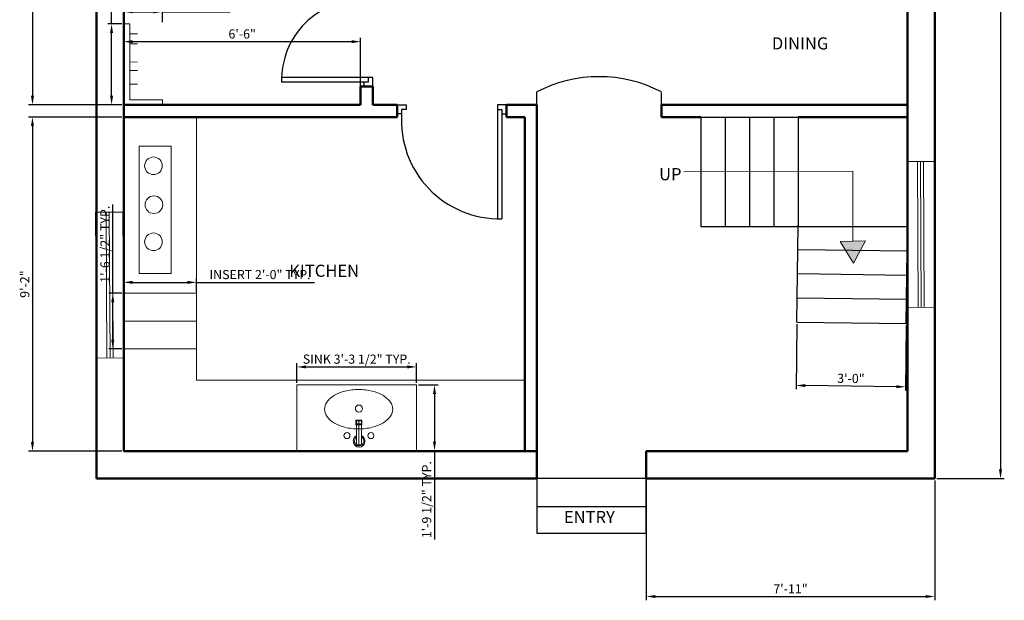
# Model space of a CAD drawing. Units: inches. Extents: x 108 to 1546, y -229 to 513.
# Tile 1 of 11: x 108 to 432, y -44 to 147. Entities that reach past the tile are written whole.
import ezdxf

# ---------------------------------------------------------------- set-up
doc = ezdxf.new("R2010")
doc.units = ezdxf.units.IN
for name, color, linetype, lineweight in [('A-ANNO-DIMS', 2, 'Continuous', 18), ('A-ANNO-SYMB', 4, 'Continuous', 18), ('A-AREA-IDEN', 4, 'Continuous', 18), ('A-EQPM', 8, 'Continuous', 18), ('A-FLOR-CBNT', 8, 'Continuous', 18), ('A-FLOR-FIXT', 9, 'Continuous', 18), ('A-FLOR-STRS', 7, 'Continuous', 25), ('door', 1, 'Continuous', 25), ('wall', 7, 'Continuous', 50), ('WINDOW', 212, 'Continuous', 18)]:
    doc.layers.add(name, color=color, linetype=linetype, lineweight=lineweight)
doc.styles.get("Standard").update_dxf_attribs({"font": 'arial.ttf'})
doc.dimstyles.new('ISO-25', dxfattribs={"dimtxt": 3, "dimasz": 3, "dimexe": 1.25, "dimexo": 0.625, "dimtad": 1, "dimdec": 1, "dimlunit": 3, "dimtxsty": 'Standard', "dimcen": 2.5, "dimadec": 0, "dimazin": 0, "dimtfac": 1, "dimtdec": 1, "dimtmove": 0, "dimatfit": 3, "dimfxl": 1, "dimarcsym": 0})

# ---------------------------------------------------------------- blocks, each defined once
blk = doc.blocks.new('A$C50A015BB')
for p, q in [((0, 0.55), (1, 0.55)), ((0, 0.55), (0, 0)), ((0.4985, 0.5), (0.5385, 0.5)), ((0.4985, 0.5), (0.4985, 0.3)), ((0.5185, 0.5), (0.5185, 0.3)), ((0.5385, 0.5), (0.5385, 0.3)), ((1, 0.55), (1, 0)), ((0.4935, 0.335), (0.4935, 0.295)), ((0.4935, 0.335), (0.5435, 0.335)), ((0.5435, 0.335), (0.5435, 0.295)), ((0.4935, 0.295), (0.5435, 0.295)), ((0.4985, 0.325), (0.5385, 0.325)), ((0.4985, 0.3), (0.5385, 0.3)), ((0, 0), (1, 0)), ((0, 0), (1, 0))]:
    blk.add_line(p, q)
for centre, radius in [((0.4185, 0.424), 0.025), ((0.6185, 0.424), 0.025), ((0.5185, 0.1981), 0.0298)]:
    blk.add_circle(centre, radius)
for centre, radius, start, end in [((0.5201, 0.4703), 0.0497, 291.74253, 244.23308), ((0.5201, 0.4703), 0.0397, 297.63203, 237.02558), ((0.4772, 0.0383), 0.3252, 103.48533, 120.06859), ((0.5157, -0.1225), 0.4906, 90, 103.48533), ((0.5157, -0.1225), 0.4906, 76.51467, 90), ((0.5543, 0.0383), 0.3252, 59.93141, 76.51467), ((0.3299, 0.2031), 0.0991, 144.41781, 180), ((0.4185, 0.1397), 0.2081, 120.06859, 144.41781), ((0.613, 0.1397), 0.2081, 35.58219, 59.93141), ((0.7016, 0.2031), 0.0991, 0, 35.58219), ((0.3299, 0.2031), 0.0991, 180, 215.58219), ((0.7016, 0.2031), 0.0991, 324.41781, 0), ((0.4185, 0.2665), 0.2081, 215.58219, 239.93141), ((0.4772, 0.3679), 0.3252, 239.93141, 256.51467), ((0.5543, 0.3679), 0.3252, 283.48533, 300.06859), ((0.613, 0.2665), 0.2081, 300.06859, 324.41781), ((0.5157, 0.5288), 0.4906, 256.51467, 270), ((0.5157, 0.5288), 0.4906, 270, 283.48533)]:
    blk.add_arc(centre, radius, start, end)
blk = doc.blocks.new('*D22')
at = {"layer": 'A-ANNO-DIMS', "color": 0, "lineweight": -2, "transparency": 16777216}
for p, q in [((409.55, 356.47), (431.8, 356.47)), ((430.55, 353.47), (430.55, -0.53)), ((409.55, -3.53), (431.8, -3.53))]:
    blk.add_line(p, q, dxfattribs=at)
at = {"layer": 'A-ANNO-DIMS', "color": 0, "transparency": 16777216}
for points in [[(430.05, 353.47), (431.05, 353.47), (430.55, 356.47)], [(430.05, -0.53), (431.05, -0.53), (430.55, -3.53)]]:
    blk.add_solid(points, dxfattribs=at)
at = {"layer": 'Defpoints', "color": 0, "transparency": 16777216}
for p in [(408.92, 356.47), (408.92, -3.53), (430.55, -3.53)]:
    blk.add_point(p, dxfattribs=at)
at = {"layer": 'A-ANNO-DIMS', "color": 0, "transparency": 16777216, "insert": (428.39, 176.47), "char_height": 3, "attachment_point": 5, "rotation": 90}
blk.add_mtext("30'", dxfattribs=at)
blk = doc.blocks.new('WINDOW-48X9')
for p, q in [((0, 9), (0, 0)), ((0, 9), (48, 9)), ((48, 9), (48, 0)), ((0, 5.5), (48, 5.5)), ((0, 4.5), (48, 4.5)), ((0, 3.5), (48, 3.5)), ((0, 0), (48, 0))]:
    blk.add_line(p, q)
blk = doc.blocks.new('DOOR-SWING-36')
for p, q in [((1.5, 1.5), (1.5, 37.5)), ((3, 1.5), (3, 37.5)), ((0, 3), (0, 0)), ((1.5, 3), (0, 3)), ((1.5, 1.5), (1.5, 3)), ((3, 1.5), (1.5, 1.5)), ((3, 0), (3, 1.5)), ((33, 0), (33, 1.5)), ((33, 1.5), (34.5, 1.5)), ((34.5, 1.5), (34.5, 3)), ((34.5, 3), (36, 3)), ((36, 3), (36, 0)), ((0, 0), (3, 0)), ((36, 0), (33, 0))]:
    blk.add_line(p, q)
blk.add_arc((2.25, 5.18), 32.32, 356.1244, 91.3295)
blk = doc.blocks.new('DOOR-SWING-30')
for p, q in [((27, 30), (30, 30)), ((27, 28.5), (27, 30)), ((30, 30), (30, 27)), ((28.5, 28.5), (27, 28.5)), ((28.5, 27), (28.5, 28.5)), ((30, 27), (28.5, 27)), ((30, 3), (0, 3)), ((28.5, 1.5), (0, 1.5)), ((28.5, 1.5), (27, 1.5)), ((27, 1.5), (27, 0)), ((30, 3), (28.5, 3)), ((28.5, 3), (28.5, 1.5)), ((30, 0), (30, 3)), ((27, 0), (30, 0))]:
    blk.add_line(p, q)
blk.add_arc((26.25, 2.25), 26.26, 88.3634, 181.6366)
blk = doc.blocks.new('COOKTOP-3-BURNER')
blk.add_lwpolyline([(0, 41.89), (10.48, 41.89), (10.48, 0), (0, 0)], close=True)
for centre in [(4.66, 35.46), (4.81, 22.66), (4.66, 10.45)]:
    blk.add_circle(centre, 2.9)
blk = doc.blocks.new('COUNTER-INSERT-DIVIDED')
blk.add_line((0, 9.14), (23.96, 9.14))
blk.add_lwpolyline([(0, 18.28), (23.96, 18.28), (23.96, 0), (0, 0)], close=True)
blk = doc.blocks.new('ENTRY-STEPS-36')
for p, q in [((0, 8.79), (36, 8.79)), ((0, 0), (36, 0))]:
    blk.add_line(p, q)
blk.add_lwpolyline([(36, 0), (36, 18), (0, 18), (0, 0)])
blk = doc.blocks.new('BATH-CORNER-RACK')
for p, q in [((2.03, 23.32), (4.51, 23.38)), ((2.03, 20.06), (4.51, 20.12)), ((2.03, 14.08), (4.51, 14.14)), ((2.03, 11.27), (4.51, 11.33)), ((2.03, 6.76), (4.51, 6.83))]:
    blk.add_line(p, q)
for points in [[(2.03, 1.66), (2.03, 26.63), (0, 26.63), (0, 0), (2.03, 0)], [(0, 1.66), (0, 1.66), (0, 0), (12.78, 0), (12.78, 1.66), (2.03, 1.66)]]:
    blk.add_lwpolyline(points)
blk = doc.blocks.new('*D56')
at = {"layer": 'A-ANNO-DIMS', "color": 0, "lineweight": -2, "transparency": 16777216}
for p, q in [((198.95, 27.94), (198.95, 34.47)), ((201.95, 33.22), (235.32, 33.22)), ((238.32, 27.94), (238.32, 34.47))]:
    blk.add_line(p, q, dxfattribs=at)
at = {"layer": 'A-ANNO-DIMS', "color": 0, "transparency": 16777216}
for points in [[(201.95, 33.72), (201.95, 32.72), (198.95, 33.22)], [(235.32, 33.72), (235.32, 32.72), (238.32, 33.22)]]:
    blk.add_solid(points, dxfattribs=at)
at = {"layer": 'Defpoints', "color": 0, "transparency": 16777216}
for p in [(238.32, 33.22), (198.95, 27.31), (238.32, 27.31)]:
    blk.add_point(p, dxfattribs=at)
at = {"layer": 'A-ANNO-DIMS', "color": 0, "transparency": 16777216, "insert": (218.64, 35.39), "char_height": 3, "attachment_point": 5}
blk.add_mtext('SINK 3\'-3 1/2" TYP.', dxfattribs=at)
blk = doc.blocks.new('*D57')
at = {"layer": 'A-ANNO-DIMS', "color": 0, "lineweight": -2, "transparency": 16777216}
for p, q in [((238.95, 27.31), (245.48, 27.31)), ((244.23, 24.31), (244.23, 8.66)), ((238.95, 5.66), (245.48, 5.66)), ((244.23, 5.66), (244.23, -23.59))]:
    blk.add_line(p, q, dxfattribs=at)
at = {"layer": 'A-ANNO-DIMS', "color": 0, "transparency": 16777216}
for points in [[(243.73, 24.31), (244.73, 24.31), (244.23, 27.31)], [(243.73, 8.66), (244.73, 8.66), (244.23, 5.66)]]:
    blk.add_solid(points, dxfattribs=at)
at = {"layer": 'Defpoints', "color": 0, "transparency": 16777216}
for p in [(238.32, 27.31), (238.32, 5.66), (244.23, 5.66)]:
    blk.add_point(p, dxfattribs=at)
at = {"layer": 'A-ANNO-DIMS', "color": 0, "transparency": 16777216, "insert": (242.05, -10.47), "char_height": 3, "attachment_point": 5, "rotation": 90}
blk.add_mtext('1\'-9 1/2" TYP.', dxfattribs=at)
blk = doc.blocks.new('*D64')
at = {"layer": 'A-ANNO-DIMS', "color": 0, "lineweight": -2, "transparency": 16777216}
for p, q in [((141.92, 58.09), (141.92, 62.31)), ((165.89, 58.09), (165.89, 62.31)), ((144.92, 61.06), (162.89, 61.06)), ((165.89, 61.06), (204.74, 61.06))]:
    blk.add_line(p, q, dxfattribs=at)
at = {"layer": 'A-ANNO-DIMS', "color": 0, "transparency": 16777216}
for points in [[(144.92, 61.56), (144.92, 60.56), (141.92, 61.06)], [(162.89, 61.56), (162.89, 60.56), (165.89, 61.06)]]:
    blk.add_solid(points, dxfattribs=at)
at = {"layer": 'Defpoints', "color": 0, "transparency": 16777216}
for p in [(165.89, 61.06), (141.92, 57.46), (165.89, 57.46)]:
    blk.add_point(p, dxfattribs=at)
at = {"layer": 'A-ANNO-DIMS', "color": 0, "transparency": 16777216, "insert": (186.81, 63.23), "char_height": 3, "attachment_point": 5}
blk.add_mtext('INSERT 2\'-0" TYP.', dxfattribs=at)
blk = doc.blocks.new('*D65')
at = {"layer": 'A-ANNO-DIMS', "color": 0, "lineweight": -2, "transparency": 16777216}
for p, q in [((138.33, 57.46), (138.33, 86.71)), ((141.3, 57.46), (137.08, 57.46)), ((138.33, 42.18), (138.33, 54.46)), ((141.3, 39.18), (137.08, 39.18))]:
    blk.add_line(p, q, dxfattribs=at)
at = {"layer": 'A-ANNO-DIMS', "color": 0, "transparency": 16777216}
for points in [[(137.83, 54.46), (138.83, 54.46), (138.33, 57.46)], [(137.83, 42.18), (138.83, 42.18), (138.33, 39.18)]]:
    blk.add_solid(points, dxfattribs=at)
at = {"layer": 'Defpoints', "color": 0, "transparency": 16777216}
for p in [(138.33, 57.46), (141.92, 57.46), (141.92, 39.18)]:
    blk.add_point(p, dxfattribs=at)
at = {"layer": 'A-ANNO-DIMS', "color": 0, "transparency": 16777216, "insert": (136.15, 73.59), "char_height": 3, "attachment_point": 5, "rotation": 90}
blk.add_mtext('1\'-6 1/2" TYP.', dxfattribs=at)
blk = doc.blocks.new('*D68')
at = {"layer": 'A-ANNO-DIMS', "color": 0, "lineweight": -2, "transparency": 16777216}
for p, q in [((137.93, 146.1), (137.93, 188.28)), ((141.3, 146.1), (136.68, 146.1)), ((137.93, 122.47), (137.93, 143.1)), ((141.3, 119.47), (136.68, 119.47))]:
    blk.add_line(p, q, dxfattribs=at)
at = {"layer": 'A-ANNO-DIMS', "color": 0, "transparency": 16777216}
for points in [[(137.43, 143.1), (138.43, 143.1), (137.93, 146.1)], [(137.43, 122.47), (138.43, 122.47), (137.93, 119.47)]]:
    blk.add_solid(points, dxfattribs=at)
at = {"layer": 'Defpoints', "color": 0, "transparency": 16777216}
for p in [(137.93, 146.1), (141.92, 146.1), (141.92, 119.47)]:
    blk.add_point(p, dxfattribs=at)
at = {"layer": 'A-ANNO-DIMS', "color": 0, "transparency": 16777216, "insert": (135.75, 168.69), "char_height": 3, "attachment_point": 5, "rotation": 90}
blk.add_mtext('RACK 2\'-2 1/2" TYP.', dxfattribs=at)
blk = doc.blocks.new('*D69')
at = {"layer": 'A-ANNO-DIMS', "color": 0, "lineweight": -2, "transparency": 16777216}
for p, q in [((141.92, 146.72), (141.92, 151.34)), ((144.92, 150.09), (151.7, 150.09)), ((154.7, 146.72), (154.7, 151.34)), ((154.7, 150.09), (176.96, 150.09))]:
    blk.add_line(p, q, dxfattribs=at)
at = {"layer": 'A-ANNO-DIMS', "color": 0, "transparency": 16777216}
for points in [[(144.92, 150.59), (144.92, 149.59), (141.92, 150.09)], [(151.7, 150.59), (151.7, 149.59), (154.7, 150.09)]]:
    blk.add_solid(points, dxfattribs=at)
at = {"layer": 'Defpoints', "color": 0, "transparency": 16777216}
for p in [(154.7, 150.09), (141.92, 146.1), (154.7, 146.1)]:
    blk.add_point(p, dxfattribs=at)
at = {"layer": 'A-ANNO-DIMS', "color": 0, "transparency": 16777216, "insert": (167.33, 152.22), "char_height": 3, "attachment_point": 5}
blk.add_mtext('1\'-1" TYP.', dxfattribs=at)
blk = doc.blocks.new('*D74')
at = {"layer": 'A-ANNO-DIMS', "color": 0, "lineweight": -2, "transparency": 16777216}
for p, q in [((141.92, 120.09), (141.92, 141.52)), ((144.92, 140.27), (216.92, 140.27)), ((219.92, 120.09), (219.92, 141.52))]:
    blk.add_line(p, q, dxfattribs=at)
at = {"layer": 'A-ANNO-DIMS', "color": 0, "transparency": 16777216}
for points in [[(144.92, 140.77), (144.92, 139.77), (141.92, 140.27)], [(216.92, 140.77), (216.92, 139.77), (219.92, 140.27)]]:
    blk.add_solid(points, dxfattribs=at)
at = {"layer": 'Defpoints', "color": 0, "transparency": 16777216}
for p in [(219.92, 140.27), (141.92, 119.47), (219.92, 119.47)]:
    blk.add_point(p, dxfattribs=at)
at = {"layer": 'A-ANNO-DIMS', "color": 0, "transparency": 16777216, "insert": (180.92, 142.43), "char_height": 3, "attachment_point": 5}
blk.add_mtext('6\'-6"', dxfattribs=at)
blk = doc.blocks.new('*D75')
at = {"layer": 'A-ANNO-DIMS', "color": 0, "lineweight": -2, "transparency": 16777216}
for p, q in [((313.92, -4.16), (313.92, -43.58)), ((408.92, -4.16), (408.92, -43.58)), ((316.92, -42.33), (405.92, -42.33))]:
    blk.add_line(p, q, dxfattribs=at)
at = {"layer": 'A-ANNO-DIMS', "color": 0, "transparency": 16777216}
for points in [[(316.92, -41.83), (316.92, -42.83), (313.92, -42.33)], [(405.92, -41.83), (405.92, -42.83), (408.92, -42.33)]]:
    blk.add_solid(points, dxfattribs=at)
at = {"layer": 'Defpoints', "color": 0, "transparency": 16777216}
for p in [(313.92, -3.53), (408.92, -3.53), (408.92, -42.33)]:
    blk.add_point(p, dxfattribs=at)
at = {"layer": 'A-ANNO-DIMS', "color": 0, "transparency": 16777216, "insert": (361.42, -40.2), "char_height": 3, "attachment_point": 5}
blk.add_mtext('7\'-11"', dxfattribs=at)
blk = doc.blocks.new('*D77')
at = {"layer": 'A-ANNO-DIMS', "color": 0, "lineweight": -2, "transparency": 16777216}
for p, q in [((141.3, 211.47), (110.64, 211.47)), ((111.89, 208.47), (111.89, 122.47)), ((141.3, 119.47), (110.64, 119.47))]:
    blk.add_line(p, q, dxfattribs=at)
at = {"layer": 'A-ANNO-DIMS', "color": 0, "transparency": 16777216}
for points in [[(111.39, 208.47), (112.39, 208.47), (111.89, 211.47)], [(111.39, 122.47), (112.39, 122.47), (111.89, 119.47)]]:
    blk.add_solid(points, dxfattribs=at)
at = {"layer": 'Defpoints', "color": 0, "transparency": 16777216}
for p in [(141.92, 211.47), (111.89, 119.47), (141.92, 119.47)]:
    blk.add_point(p, dxfattribs=at)
at = {"layer": 'A-ANNO-DIMS', "color": 0, "transparency": 16777216, "insert": (109.73, 165.47), "char_height": 3, "attachment_point": 5, "rotation": 90}
blk.add_mtext('7\'-8"', dxfattribs=at)
blk = doc.blocks.new('*D78')
at = {"layer": 'A-ANNO-DIMS', "color": 0, "lineweight": -2, "transparency": 16777216}
for p, q in [((141.3, 115.47), (110.64, 115.47)), ((111.89, 112.47), (111.89, 8.47)), ((141.3, 5.47), (110.64, 5.47))]:
    blk.add_line(p, q, dxfattribs=at)
at = {"layer": 'A-ANNO-DIMS', "color": 0, "transparency": 16777216}
for points in [[(111.39, 112.47), (112.39, 112.47), (111.89, 115.47)], [(111.39, 8.47), (112.39, 8.47), (111.89, 5.47)]]:
    blk.add_solid(points, dxfattribs=at)
at = {"layer": 'Defpoints', "color": 0, "transparency": 16777216}
for p in [(141.92, 115.47), (111.89, 5.47), (141.92, 5.47)]:
    blk.add_point(p, dxfattribs=at)
at = {"layer": 'A-ANNO-DIMS', "color": 0, "transparency": 16777216, "insert": (109.73, 60.47), "char_height": 3, "attachment_point": 5, "rotation": 90}
blk.add_mtext('9\'-2"', dxfattribs=at)
blk = doc.blocks.new('*D79')
at = {"layer": 'A-ANNO-DIMS', "color": 0, "lineweight": -2, "transparency": 16777216}
for p, q in [((363.52, 47.29), (363.26, 25.87)), ((399.52, 46.85), (399.25, 25.42)), ((396.27, 26.71), (366.27, 27.08))]:
    blk.add_line(p, q, dxfattribs=at)
at = {"layer": 'A-ANNO-DIMS', "color": 0, "transparency": 16777216}
for points in [[(366.28, 27.58), (366.27, 26.58), (363.27, 27.12)], [(396.28, 27.21), (396.26, 26.21), (399.27, 26.67)]]:
    blk.add_solid(points, dxfattribs=at)
at = {"layer": 'Defpoints', "color": 0, "transparency": 16777216}
for p in [(363.53, 47.92), (399.53, 47.47), (363.27, 27.12)]:
    blk.add_point(p, dxfattribs=at)
at = {"layer": 'A-ANNO-DIMS', "color": 0, "transparency": 16777216, "insert": (381.3, 29.05), "char_height": 3, "attachment_point": 5, "rotation": 359.2923}
blk.add_mtext('3\'-0"', dxfattribs=at)

msp = doc.modelspace()

# ---------------------------------------------------------------- hatches: boundary and pattern name
at = {"layer": 'A-ANNO-SYMB'}
h = msp.add_hatch(color=256, dxfattribs=at)
h.dxf.hatch_style = 1
h.paths.add_polyline_path([(386.1, 74.76), (377.74, 74.46), (379.46, 71.72), (384.46, 71.66)])
h.paths.add_polyline_path([(384.46, 71.66), (379.46, 71.72), (382.19, 67.37)])

# ---------------------------------------------------------------- linework, layer by layer
for p, q in [((326.29, 97.47), (381.92, 97.65)), ((381.92, 97.65), (381.92, 74.61))]:
    msp.add_line(p, q, dxfattribs=at)
msp.add_lwpolyline([(382.19, 67.37), (386.1, 74.76), (377.74, 74.46)], close=True, dxfattribs=at)
at = {"layer": 'A-FLOR-CBNT'}
for p, q in [((141.92, 115.47), (165.89, 115.47)), ((141.92, 5.47), (141.92, 115.47)), ((165.89, 115.47), (165.89, 28.9)), ((141.92, 28.9), (141.92, 5.47)), ((273.92, 28.9), (165.89, 28.9)), ((273.92, 5.47), (273.92, 28.9)), ((165.89, 5.47), (141.92, 5.47)), ((141.92, 5.47), (273.92, 5.47))]:
    msp.add_line(p, q, dxfattribs=at)
at = {"layer": 'A-FLOR-FIXT'}
msp.add_line((143.95, 142.79), (143.95, 142.79), dxfattribs=at)
at = {"layer": 'A-FLOR-STRS'}
for p, q in [((331.92, 115.47), (331.92, 79.47)), ((331.92, 115.47), (363.92, 115.47)), ((339.92, 115.47), (339.92, 79.47)), ((347.92, 115.47), (347.92, 79.47)), ((355.92, 115.47), (355.92, 79.47)), ((399.92, 115.47), (363.92, 115.47)), ((363.92, 115.47), (363.92, 79.47)), ((399.92, 79.47), (399.92, 115.47)), ((331.92, 79.47), (363.92, 79.47)), ((363.53, 47.92), (363.92, 79.91)), ((363.92, 79.47), (399.92, 79.47)), ((399.53, 47.47), (399.92, 79.47)), ((363.83, 71.92), (399.82, 71.47)), ((363.73, 63.92), (399.72, 63.47)), ((363.63, 55.92), (399.63, 55.47)), ((363.53, 47.92), (399.53, 47.47))]:
    msp.add_line(p, q, dxfattribs=at)
at = {"layer": 'door'}
for p, q in [((277.92, 119.47), (277.92, 123.71)), ((318.92, 119.47), (318.92, 123.53))]:
    msp.add_line(p, q, dxfattribs=at)
msp.add_arc((298.42, 84.53), 44.21, 62.3775, 117.6225, dxfattribs=at)
at = {"layer": 'wall'}
for p, q in [((132.92, 356.47), (132.92, -3.53)), ((408.92, -3.53), (408.92, 356.47)), ((141.92, 347.47), (141.92, 5.47)), ((399.92, 5.47), (399.92, 347.47)), ((219.92, 125.47), (223.92, 125.47)), ((219.92, 125.47), (219.92, 119.47)), ((223.92, 125.47), (223.92, 119.47)), ((219.92, 119.47), (141.92, 119.47)), ((231.92, 119.47), (223.92, 119.47)), ((231.92, 115.47), (231.92, 119.47)), ((277.92, 119.47), (267.92, 119.47)), ((267.92, 115.47), (267.92, 119.47)), ((277.92, 119.47), (277.92, 5.47)), ((399.92, 119.47), (318.92, 119.47)), ((318.92, 115.47), (318.92, 119.47)), ((231.92, 115.47), (141.92, 115.47)), ((273.92, 115.47), (267.92, 115.47)), ((273.92, 115.47), (273.92, 5.47)), ((331.92, 115.47), (318.92, 115.47)), ((399.92, 115.47), (363.92, 115.47)), ((141.92, 5.47), (277.92, 5.47)), ((277.92, 5.47), (277.92, -3.53)), ((313.92, 5.47), (313.92, -3.53)), ((313.92, 5.47), (399.92, 5.47)), ((132.92, -3.53), (277.92, -3.53)), ((313.92, -3.53), (408.92, -3.53))]:
    msp.add_line(p, q, dxfattribs=at)

# ---------------------------------------------------------------- block references
at = {"layer": 'A-EQPM'}
msp.add_blockref('COOKTOP-3-BURNER', (147.06, 63.95), dxfattribs=at)
at = {"layer": 'A-FLOR-CBNT'}
msp.add_blockref('COUNTER-INSERT-DIVIDED', (141.92, 39.18), dxfattribs=at)
at = {"layer": 'A-FLOR-FIXT'}
msp.add_blockref('BATH-CORNER-RACK', (141.92, 119.47), dxfattribs=at)
at = {"layer": 'A-FLOR-FIXT', "xscale": -39.37007874015748, "yscale": 39.37007874015748, "zscale": 39.37007874015748, "rotation": 180}
msp.add_blockref('A$C50A015BB', (198.95, 27.31), dxfattribs=at)
at = {"layer": 'A-FLOR-STRS'}
msp.add_blockref('ENTRY-STEPS-36', (277.92, -21.53), dxfattribs=at)
at = {"layer": 'door'}
msp.add_blockref('DOOR-SWING-30', (193.92, 125.47), dxfattribs=at)
at = {"layer": 'door', "rotation": 180}
msp.add_blockref('DOOR-SWING-36', (267.92, 119.47), dxfattribs=at)
at = {"layer": 'WINDOW'}
for p, rotation in [((408.92, 52.84), 90.27995600981023), ((141.92, 36.2), 90.2799560098106)]:
    msp.add_blockref('WINDOW-48X9', p, dxfattribs=dict(at, rotation=rotation))

# ---------------------------------------------------------------- texts
at = {"layer": 'A-ANNO-SYMB', "insert": (318.15, 98.66), "char_height": 4, "attachment_point": 1}
msp.add_mtext_dynamic_manual_height_columns('UP', width=57.4311, gutter_width=12.5, heights=[12.84], dxfattribs=at)
at = {"layer": 'A-AREA-IDEN', "char_height": 4, "attachment_point": 1}
for s, insert in [('DINING', (355.28, 141.69)), ('KITCHEN', (196.42, 66.87)), ('ENTRY', (286.82, -14.18))]:
    msp.add_mtext_dynamic_manual_height_columns(s, width=57.4311, gutter_width=12.5, heights=[12.84], dxfattribs=dict(at, insert=insert))

# ---------------------------------------------------------------- dimensions: what is measured, and where the dimension line sits
at = {"layer": 'A-ANNO-DIMS'}
for base, p1, p2, angle, override, picture, middle in [((430.55, -3.53), (408.92, 356.47), (408.92, -3.53), 90, {"dimclrd": 0, "dimclre": 0, "dimclrt": 0}, '*D22', (428.39, 176.47)), ((111.89, 119.47), (141.92, 211.47), (141.92, 119.47), 90, {"dimdec": 1, "dimlfac": 1, "dimrnd": 0, "dimzin": 1, "dimdsep": 46, "dimlunit": 4, "dimfrac": 2}, '*D77', (109.73, 165.47)), ((219.92, 140.27), (141.92, 119.47), (219.92, 119.47), 0, {"dimdec": 1, "dimlfac": 1, "dimrnd": 0, "dimzin": 1, "dimdsep": 46, "dimlunit": 4, "dimfrac": 2}, '*D74', (180.92, 142.43)), ((111.89, 5.47), (141.92, 115.47), (141.92, 5.47), 90, {"dimdec": 1, "dimlfac": 1, "dimrnd": 0, "dimzin": 1, "dimdsep": 46, "dimlunit": 4, "dimfrac": 2}, '*D78', (109.73, 60.47)), ((363.27, 27.12), (399.53, 47.47), (363.53, 47.92), 179.2923, {"dimdec": 1, "dimlfac": 1, "dimrnd": 0, "dimzin": 1, "dimdsep": 46, "dimlunit": 4, "dimfrac": 2}, '*D79', (381.3, 29.05))]:
    dim = msp.add_linear_dim(base=base, p1=p1, p2=p2, angle=angle, dimstyle='ISO-25', override=override, dxfattribs=at)
    dim.commit()
    dim.dimension.update_dxf_attribs({"geometry": picture, "text_midpoint": middle})
for base, p1, p2, angle, text, picture, middle in [((137.93, 146.1), (141.92, 119.47), (141.92, 146.1), 90, 'RACK <> TYP.', '*D68', (135.75, 168.69)), ((138.33, 57.46), (141.92, 39.18), (141.92, 57.46), 90, '<> TYP.', '*D65', (136.15, 73.59)), ((244.2283, 5.657), (238.3227, 27.3106), (238.3227, 5.657), 270, '<> TYP.', '*D57', (242.0521, -10.4652))]:
    dim = msp.add_linear_dim(base=base, p1=p1, p2=p2, angle=angle, text=text, dimstyle='ISO-25', override={"dimdec": 1, "dimlfac": 1, "dimrnd": 0, "dimzin": 1, "dimdsep": 46, "dimlunit": 4, "dimfrac": 2}, dxfattribs=at)
    dim.commit()
    dim.dimension.update_dxf_attribs({"geometry": picture, "text_midpoint": middle})
for base, p1, p2, text, picture, middle in [((154.7, 150.09), (141.92, 146.1), (154.7, 146.1), '<> TYP.', '*D69', (167.33, 152.22)), ((165.89, 61.06), (141.92, 57.46), (165.89, 57.46), 'INSERT <> TYP.', '*D64', (186.81, 63.23)), ((238.32, 33.22), (198.95, 27.31), (238.32, 27.31), 'SINK <> TYP.', '*D56', (218.64, 35.39))]:
    dim = msp.add_linear_dim(base=base, p1=p1, p2=p2, text=text, dimstyle='ISO-25', override={"dimdec": 1, "dimlfac": 1, "dimrnd": 0, "dimzin": 1, "dimdsep": 46, "dimlunit": 4, "dimfrac": 2}, dxfattribs=at)
    dim.commit()
    dim.dimension.update_dxf_attribs({"geometry": picture, "text_midpoint": middle})
dim = msp.add_linear_dim(base=(408.92, -42.33), p1=(313.92, -3.53), p2=(408.92, -3.53), dimstyle='ISO-25', override={"dimdec": 1, "dimlfac": 1, "dimrnd": 0, "dimzin": 1, "dimdsep": 46, "dimlunit": 4, "dimfrac": 2}, dxfattribs=at)
dim.commit()
dim.dimension.update_dxf_attribs({"geometry": '*D75', "text_midpoint": (361.42, -40.2)})

doc.saveas('drawing.dxf')
